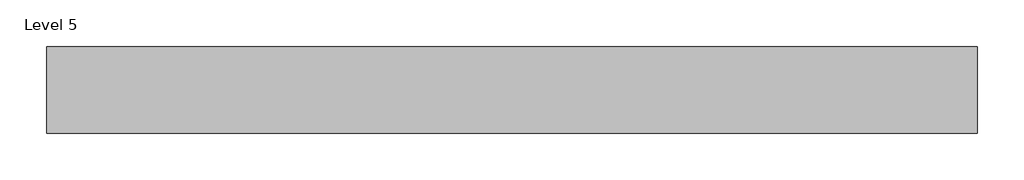
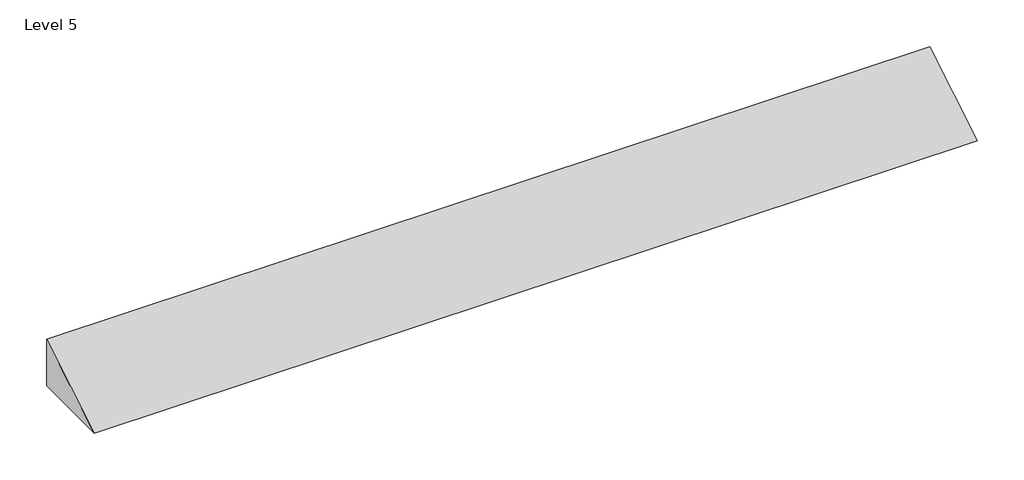
# One storey: 1 proxy.
"""IFC4 building model written with IfcOpenShell, lengths in millimetres."""

from ifc_helpers import new_model, si_unit, origin, place, context, project, spatial, transform, mapped, element, save
from components import generic_models_1_generic_models_1_2c9bbbb1

model = new_model("IFC4")

# Units and contexts
model_context = context("Model", 3, world=origin())
ifc_project = project(units=[si_unit("LENGTHUNIT", "METRE", prefix="MILLI")], contexts=[model_context])

# Site, building, storey
site = spatial("IfcSite", under=ifc_project)
building = spatial("IfcBuilding", under=site)
storey = spatial("IfcBuildingStorey", under=building, Name="Level 5", Elevation=-304.8)

# Proxy
placement = place(None, origin())
generic_models_1_generic_models_1_shape = generic_models_1_generic_models_1_2c9bbbb1(model_context)
element("IfcBuildingElementProxy", 1, Name="Generic Models 1 : Generic Models 1", ObjectType="Generic Models 1 : Generic Models 1", at=placement, inside=storey, context=model_context, shape_type="MappedRepresentation", body=[
    mapped(generic_models_1_generic_models_1_shape, transform((0.0, 0.0, 0.0), x_axis=(1.0, 0.0, 0.0), y_axis=(0.0, 1.0, 0.0), z_axis=(0.0, 0.0, 1.0))),
])

save(model, "model.ifc")

# Revit data of these elements
# Element 1 (IfcBuildingElementProxy, "Generic Models 1 : Generic Models 1")
#   Phase Created = New Construction
#   Materials on its faces: "DARK WALNUT COLOUR"
# Materials
#   "DARK WALNUT COLOUR": class "Generic", colour RGB 120 120 120, transparency 0, Cost = 0
